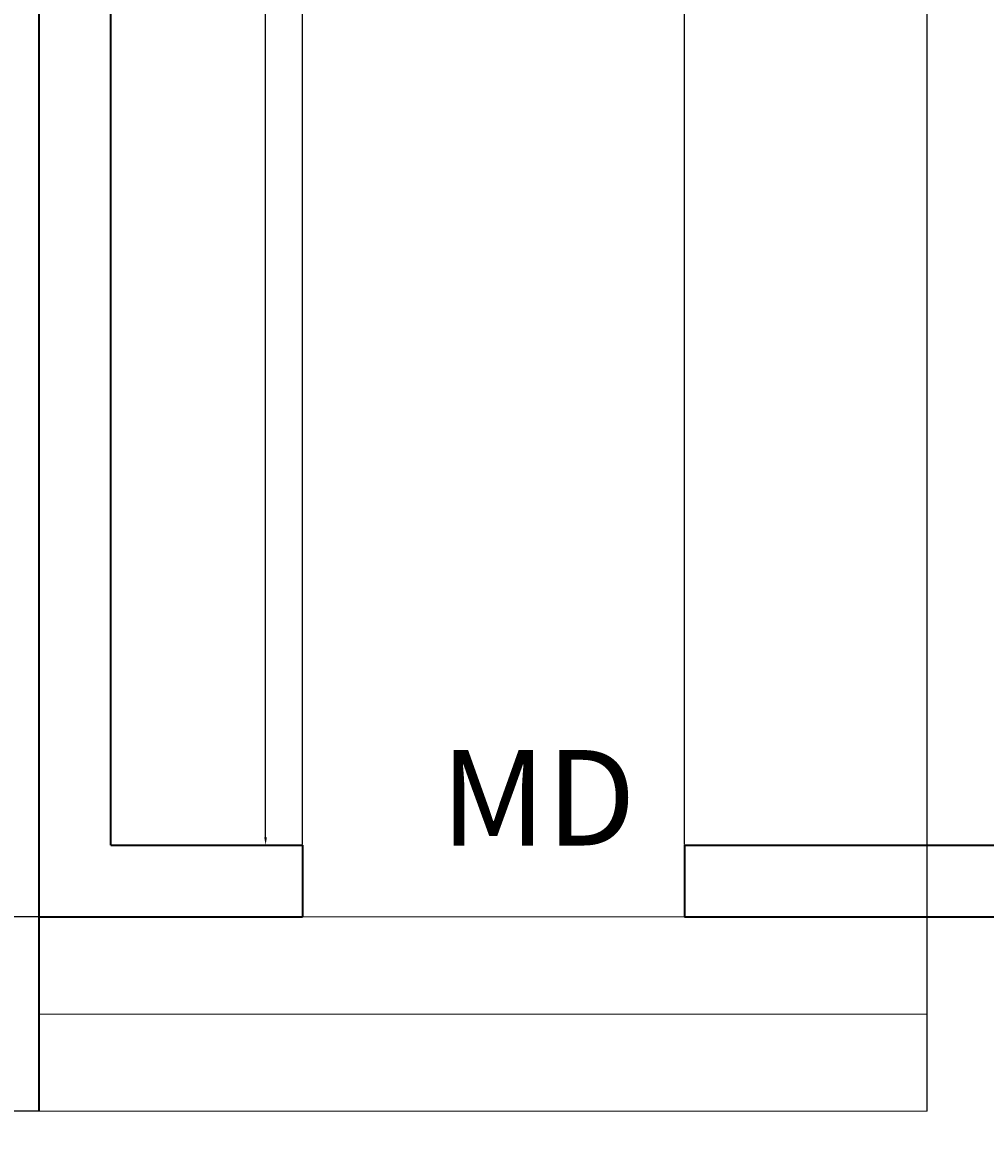
# Model space of a CAD drawing. Units: inches. Extents: x -304 to 580, y 363 to 1149.
# Tile 4 of 11: x -25 to 96, y 512 to 653. Entities that reach past the tile are written whole.
import ezdxf

# ---------------------------------------------------------------- set-up
doc = ezdxf.new("R2010")
doc.units = ezdxf.units.IN
doc.header["$MEASUREMENT"] = 0
for name, color, linetype, lineweight in [('A-ANNO-DIMS', 2, 'Continuous', 13), ('A-ANNO-IDEN', 7, 'Continuous', 18), ('A-FLOR-STRS', 40, 'Continuous', 18), ('A-WALL', 40, 'Continuous', 35)]:
    doc.layers.add(name, color=color, linetype=linetype, lineweight=lineweight)
doc.styles.get("Standard").update_dxf_attribs({"font": 'arial.ttf'})
doc.dimstyles.get("Standard").update_dxf_attribs({"dimtxt": 1, "dimasz": 1, "dimexe": 0.18, "dimexo": 0.0625, "dimgap": 0.09, "dimtad": 0, "dimtih": 1, "dimtoh": 1, "dimdec": 0, "dimzin": 0, "dimdsep": 46, "dimlunit": 3, "dimtxsty": 'Standard', "dimcen": 0.09, "dimadec": 0, "dimazin": 0, "dimtfac": 1, "dimtdec": 0, "dimtofl": 0, "dimtmove": 0, "dimatfit": 3, "dimfxl": 1, "dimtolj": 1, "dimtzin": 0, "dimarcsym": 0})

# ---------------------------------------------------------------- blocks, each defined once
blk = doc.blocks.new('*D1')
at = {"layer": 'A-ANNO-DIMS', "color": 0, "lineweight": -2, "transparency": 16777216}
for p, q in [((-22.63, 1004.95), (-237.62, 1004.95)), ((-237.44, 1003.95), (-237.44, 721.93)), ((-237.44, 402.95), (-237.44, 684.96)), ((-22.63, 401.95), (-237.62, 401.95))]:
    blk.add_line(p, q, dxfattribs=at)
at = {"layer": 'A-ANNO-DIMS', "color": 0, "transparency": 16777216}
for points in [[(-237.61, 1003.95), (-237.28, 1003.95), (-237.44, 1004.95)], [(-237.61, 402.95), (-237.28, 402.95), (-237.44, 401.95)]]:
    blk.add_solid(points, dxfattribs=at)
at = {"layer": 'Defpoints', "color": 0, "transparency": 16777216}
for p in [(-22.57, 1004.95), (-237.44, 401.95), (-22.57, 401.95)]:
    blk.add_point(p, dxfattribs=at)
at = {"layer": 'A-ANNO-DIMS', "color": 0, "transparency": 16777216, "insert": (-237.44, 703.45), "char_height": 1, "attachment_point": 5}
blk.add_mtext('\\A1;{\\H36x;50\'-3"}', dxfattribs=at)
blk = doc.blocks.new('*D3')
at = {"layer": 'A-ANNO-DIMS', "color": 0, "lineweight": -2, "transparency": 16777216}
for p, q in [((-13.51, 789.95), (6.06, 789.95)), ((5.88, 788.95), (5.88, 672.59)), ((5.88, 550.95), (5.88, 667.3)), ((-13.51, 549.95), (6.06, 549.95))]:
    blk.add_line(p, q, dxfattribs=at)
at = {"layer": 'A-ANNO-DIMS', "color": 0, "transparency": 16777216}
for points in [[(5.71, 788.95), (6.04, 788.95), (5.88, 789.95)], [(5.71, 550.95), (6.04, 550.95), (5.88, 549.95)]]:
    blk.add_solid(points, dxfattribs=at)
at = {"layer": 'Defpoints', "color": 0, "transparency": 16777216}
for p in [(-13.57, 789.95), (5.88, 789.95), (-13.57, 549.95)]:
    blk.add_point(p, dxfattribs=at)
at = {"layer": 'A-ANNO-DIMS', "color": 0, "transparency": 16777216, "insert": (5.88, 669.95), "char_height": 1, "attachment_point": 5}
blk.add_mtext("\\A1;{\\H5x;20'}", dxfattribs=at)
blk = doc.blocks.new('*D34')
at = {"layer": 'A-ANNO-DIMS', "color": 0, "lineweight": -2, "transparency": 16777216}
for p, q in [((10.51, 550.01), (10.51, 1042.88)), ((11.51, 1042.7), (33.07, 1042.7)), ((57.51, 1042.7), (35.95, 1042.7)), ((58.51, 550.01), (58.51, 1042.88))]:
    blk.add_line(p, q, dxfattribs=at)
at = {"layer": 'A-ANNO-DIMS', "color": 0, "transparency": 16777216}
for points in [[(11.51, 1042.86), (11.51, 1042.53), (10.51, 1042.7)], [(57.51, 1042.86), (57.51, 1042.53), (58.51, 1042.7)]]:
    blk.add_solid(points, dxfattribs=at)
at = {"layer": 'Defpoints', "color": 0, "transparency": 16777216}
for p in [(58.51, 1042.7), (10.51, 549.95), (58.51, 549.95)]:
    blk.add_point(p, dxfattribs=at)
at = {"layer": 'A-ANNO-DIMS', "color": 0, "transparency": 16777216, "insert": (34.51, 1042.7), "char_height": 1, "attachment_point": 5}
blk.add_mtext('\\A1;4\'-0"', dxfattribs=at)
blk = doc.blocks.new('*D35')
at = {"layer": 'A-ANNO-DIMS', "color": 0, "lineweight": -2, "transparency": 16777216}
for p, q in [((-13.57, 550.01), (-13.57, 1042.88)), ((-12.57, 1042.7), (-2.96, 1042.7)), ((9.51, 1042.7), (-0.1, 1042.7)), ((10.51, 550.01), (10.51, 1042.88))]:
    blk.add_line(p, q, dxfattribs=at)
at = {"layer": 'A-ANNO-DIMS', "color": 0, "transparency": 16777216}
for points in [[(-12.57, 1042.86), (-12.57, 1042.53), (-13.57, 1042.7)], [(9.51, 1042.86), (9.51, 1042.53), (10.51, 1042.7)]]:
    blk.add_solid(points, dxfattribs=at)
at = {"layer": 'Defpoints', "color": 0, "transparency": 16777216}
for p in [(10.51, 1042.7), (-13.57, 549.95), (10.51, 549.95)]:
    blk.add_point(p, dxfattribs=at)
at = {"layer": 'A-ANNO-DIMS', "color": 0, "transparency": 16777216, "insert": (-1.53, 1042.7), "char_height": 1, "attachment_point": 5}
blk.add_mtext('\\A1;2\'-0"', dxfattribs=at)
blk = doc.blocks.new('*D36')
at = {"layer": 'A-ANNO-DIMS', "color": 0, "lineweight": -2, "transparency": 16777216}
for p, q in [((-22.57, 516.57), (-22.57, 1042.88)), ((-21.57, 1042.7), (30.65, 1042.7)), ((88.04, 1042.7), (35.82, 1042.7)), ((89.04, 516.57), (89.04, 1042.88))]:
    blk.add_line(p, q, dxfattribs=at)
at = {"layer": 'A-ANNO-DIMS', "color": 0, "transparency": 16777216}
for points in [[(-21.57, 1042.86), (-21.57, 1042.53), (-22.57, 1042.7)], [(88.04, 1042.86), (88.04, 1042.53), (89.04, 1042.7)]]:
    blk.add_solid(points, dxfattribs=at)
at = {"layer": 'Defpoints', "color": 0, "transparency": 16777216}
for p in [(89.04, 1042.7), (-22.57, 516.51), (89.04, 516.51)]:
    blk.add_point(p, dxfattribs=at)
at = {"layer": 'A-ANNO-DIMS', "color": 0, "transparency": 16777216, "insert": (33.23, 1042.7), "char_height": 1, "attachment_point": 5}
blk.add_mtext('\\A1;9\'-3 1/2"', dxfattribs=at)
blk = doc.blocks.new('*D37')
at = {"layer": 'A-ANNO-DIMS', "color": 0, "lineweight": -2, "transparency": 16777216}
for p, q in [((-22.63, 540.95), (-108.5, 540.95)), ((-108.32, 539.95), (-108.32, 529.34)), ((-108.32, 517.51), (-108.32, 528.12)), ((-22.63, 516.51), (-108.5, 516.51))]:
    blk.add_line(p, q, dxfattribs=at)
at = {"layer": 'A-ANNO-DIMS', "color": 0, "transparency": 16777216}
for points in [[(-108.49, 539.95), (-108.15, 539.95), (-108.32, 540.95)], [(-108.49, 517.51), (-108.15, 517.51), (-108.32, 516.51)]]:
    blk.add_solid(points, dxfattribs=at)
at = {"layer": 'Defpoints', "color": 0, "transparency": 16777216}
for p in [(-108.32, 540.95), (-22.57, 540.95), (-22.57, 516.51)]:
    blk.add_point(p, dxfattribs=at)
at = {"layer": 'A-ANNO-DIMS', "color": 0, "transparency": 16777216, "insert": (-108.32, 528.73), "char_height": 1, "attachment_point": 5}
blk.add_mtext('\\A1;2\'-0 1/2"', dxfattribs=at)

msp = doc.modelspace()

# ---------------------------------------------------------------- linework, layer by layer
at = {"layer": 'A-FLOR-STRS'}
msp.add_line((-22.57, 528.73), (89.04, 528.73), dxfattribs=at)
msp.add_lwpolyline([(-22.57, 540.95), (89.04, 540.95), (89.04, 516.51), (-22.57, 516.51)], close=True, dxfattribs=at)
at = {"layer": 'A-WALL'}
for p, q in [((-22.57, 516.51), (-22.57, 1004.95)), ((-13.57, 549.95), (-13.57, 789.95)), ((-13.57, 549.95), (10.51, 549.95)), ((10.51, 549.95), (10.51, 540.95)), ((58.51, 549.95), (58.51, 540.95)), ((58.51, 549.95), (183.43, 549.95)), ((-22.57, 540.95), (10.51, 540.95)), ((58.51, 540.95), (183.43, 540.95))]:
    msp.add_line(p, q, dxfattribs=at)

# ---------------------------------------------------------------- texts
at = {"layer": 'A-ANNO-IDEN', "insert": (27.86, 561.9), "char_height": 12, "attachment_point": 1}
msp.add_mtext_dynamic_manual_height_columns('MD', width=12.3109, gutter_width=1, heights=[0], dxfattribs=at)

# ---------------------------------------------------------------- dimensions: what is measured, and where the dimension line sits
at = {"layer": 'A-ANNO-DIMS'}
for base, p1, p2, picture, middle in [((89.04, 1042.7), (-22.57, 516.51), (89.04, 516.51), '*D36', (33.23, 1042.7)), ((10.51, 1042.7), (-13.57, 549.95), (10.51, 549.95), '*D35', (-1.53, 1042.7)), ((58.51, 1042.7), (10.51, 549.95), (58.51, 549.95), '*D34', (34.51, 1042.7))]:
    dim = msp.add_linear_dim(base=base, p1=p1, p2=p2, dimstyle='Standard', override={"dimdec": 1, "dimlfac": 1, "dimrnd": 0, "dimzin": 1, "dimdsep": 46, "dimlunit": 4, "dimfrac": 2}, dxfattribs=at)
    dim.commit()
    dim.dimension.update_dxf_attribs({"geometry": picture, "text_midpoint": middle})
for base, p1, p2, text, picture, middle in [((-237.44, 401.95), (-22.57, 1004.95), (-22.57, 401.95), '{\\H36x;<>}', '*D1', (-237.44, 703.45)), ((5.88, 789.95), (-13.57, 549.95), (-13.57, 789.95), '{\\H5x;<>}', '*D3', (5.88, 669.95))]:
    dim = msp.add_linear_dim(base=base, p1=p1, p2=p2, angle=90, text=text, dimstyle='Standard', override={"dimclrd": 0, "dimclre": 0, "dimclrt": 0}, dxfattribs=at)
    dim.commit()
    dim.dimension.update_dxf_attribs({"geometry": picture, "text_midpoint": middle})
dim = msp.add_linear_dim(base=(-108.32, 540.95), p1=(-22.57, 516.51), p2=(-22.57, 540.95), angle=90, dimstyle='Standard', override={"dimdec": 1, "dimlfac": 1, "dimrnd": 0, "dimzin": 1, "dimdsep": 46, "dimlunit": 4, "dimfrac": 2}, dxfattribs=at)
dim.commit()
dim.dimension.update_dxf_attribs({"geometry": '*D37', "text_midpoint": (-108.32, 528.73)})

doc.saveas('drawing.dxf')
